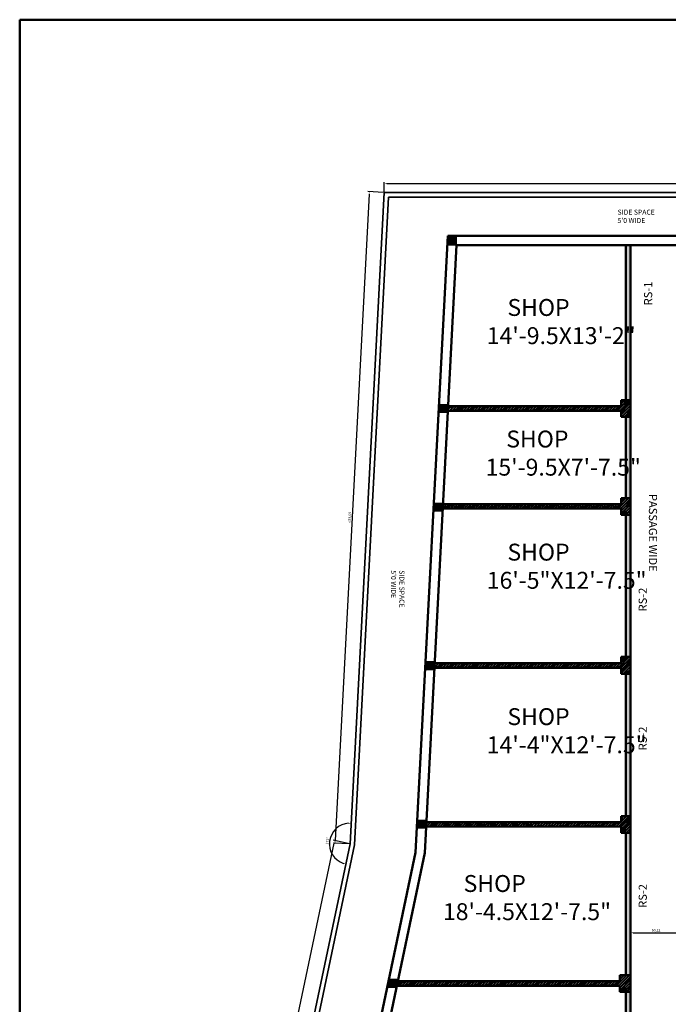
# Model space of a CAD drawing. Units: millimetres. Extents: x 2134 to 3363, y 1052 to 3233.
# Tile 6 of 11: x 2134 to 2770, y 2268 to 3233. Entities that reach past the tile are written whole.
import ezdxf

# ---------------------------------------------------------------- set-up
doc = ezdxf.new("R2010")
doc.units = ezdxf.units.MM
for name, color, linetype, lineweight in [('A-ANNO-DIMS', 2, 'Continuous', 18), ('A-ANNO-TEXT', 7, 'Continuous', 18), ('A-ANNO-TTLB', 7, 'Continuous', 50), ('A-AREA-IDEN', 3, 'Continuous', 18), ('A-COLS', 1, 'Continuous', 35), ('A-WALL', 7, 'Continuous', 50), ('A-WALL-PATT', 8, 'Continuous', 13), ('C-PROP', 6, 'Continuous', 35)]:
    doc.layers.add(name, color=color, linetype=linetype, lineweight=lineweight)
doc.styles.get("Standard").update_dxf_attribs({"font": 'arial.ttf'})
doc.styles.add('YQ_DIM', font='SUPEROS.SHX', dxfattribs={"width": 0.8, "bigfont": 'HZDX.SHX'})
doc.dimstyles.new('ISO-25', dxfattribs={"dimtxt": 2.5, "dimasz": 2.5, "dimexe": 1.25, "dimexo": 0.625, "dimtad": 1, "dimtxsty": 'Standard', "dimcen": 2.5, "dimadec": 0, "dimazin": 0, "dimtfac": 1, "dimtmove": 0, "dimatfit": 3, "dimfxl": 1, "dimarcsym": 0})
pattern_1 = [(45, (2052.4981, 1503.6934), (-1.3470384, 1.3470384), []), (45, (2053.3961, 1503.6934), (-1.3470384, 1.3470384), [])]

# ---------------------------------------------------------------- blocks, each defined once
blk = doc.blocks.new('*D7')
at = {"layer": 'A-ANNO-DIMS', "color": 0, "lineweight": -2, "transparency": 16777216}
for p, q in [((2476.99, 3062.09), (2443.78, 2428.27)), ((2491.22, 3063.85), (2475.87, 3064.66)), ((2457.74, 2425.04), (2442.4, 2425.84))]:
    blk.add_line(p, q, dxfattribs=at)
at = {"layer": 'A-ANNO-DIMS', "color": 0, "transparency": 16777216}
for points in [[(2476.58, 3062.12), (2477.41, 3062.07), (2477.12, 3064.59)], [(2443.36, 2428.3), (2444.19, 2428.25), (2443.64, 2425.78)]]:
    blk.add_solid(points, dxfattribs=at)
at = {"layer": 'Defpoints', "color": 0, "transparency": 16777216}
for p in [(2491.84, 3063.82), (2443.64, 2425.78), (2458.36, 2425.01)]:
    blk.add_point(p, dxfattribs=at)
at = {"layer": 'A-ANNO-DIMS', "color": 0, "transparency": 16777216, "insert": (2458.26, 2745.3), "char_height": 2.5, "attachment_point": 5, "rotation": 87}
blk.add_mtext('639,69', dxfattribs=at)
blk = doc.blocks.new('*D8')
at = {"layer": 'A-ANNO-DIMS', "color": 0, "lineweight": -2, "transparency": 16777216}
for p, q in [((2442.41, 2425.81), (2184.54, 1200.99)), ((2457.75, 2425.14), (2441.71, 2428.51)), ((2198.85, 1195.42), (2182.8, 1198.8))]:
    blk.add_line(p, q, dxfattribs=at)
at = {"layer": 'A-ANNO-DIMS', "color": 0, "transparency": 16777216}
for points in [[(2442.01, 2425.9), (2442.82, 2425.72), (2442.93, 2428.26)], [(2184.14, 1201.07), (2184.95, 1200.9), (2184.03, 1198.54)]]:
    blk.add_solid(points, dxfattribs=at)
at = {"layer": 'Defpoints', "color": 0, "transparency": 16777216}
for p in [(2458.36, 2425.01), (2184.03, 1198.54), (2199.46, 1195.29)]:
    blk.add_point(p, dxfattribs=at)
at = {"layer": 'A-ANNO-DIMS', "color": 0, "transparency": 16777216, "insert": (2311.4, 1813.84), "char_height": 2.5, "attachment_point": 5, "rotation": 78.11076}
blk.add_mtext('1256,67', dxfattribs=at)
blk = doc.blocks.new('*D12')
at = {"layer": 'A-ANNO-DIMS', "color": 0, "lineweight": -2, "transparency": 16777216}
for p, q in [((2733.28, 2333.03), (2733.28, 2339.03)), ((2735.78, 2337.78), (2780.9, 2337.78)), ((2783.4, 2333.03), (2783.4, 2339.03))]:
    blk.add_line(p, q, dxfattribs=at)
at = {"layer": 'A-ANNO-DIMS', "color": 0, "transparency": 16777216}
for points in [[(2735.78, 2338.2), (2735.78, 2337.36), (2733.28, 2337.78)], [(2780.9, 2338.2), (2780.9, 2337.36), (2783.4, 2337.78)]]:
    blk.add_solid(points, dxfattribs=at)
at = {"layer": 'Defpoints', "color": 0, "transparency": 16777216}
for p in [(2783.4, 2337.78), (2733.28, 2332.41), (2783.4, 2332.41)]:
    blk.add_point(p, dxfattribs=at)
at = {"layer": 'A-ANNO-DIMS', "color": 0, "transparency": 16777216, "insert": (2758.34, 2339.91), "char_height": 2.5, "attachment_point": 5}
blk.add_mtext('50,12', dxfattribs=at)
blk = doc.blocks.new('*D16')
at = {"layer": 'A-ANNO-DIMS', "color": 0, "lineweight": -2, "transparency": 16777216}
for p, q in [((2491.84, 3064.45), (2491.84, 3073.74)), ((2494.34, 3072.49), (3166.34, 3072.49)), ((3168.84, 3064.45), (3168.84, 3073.74))]:
    blk.add_line(p, q, dxfattribs=at)
at = {"layer": 'A-ANNO-DIMS', "color": 0, "transparency": 16777216}
for points in [[(2494.34, 3072.9), (2494.34, 3072.07), (2491.84, 3072.49)], [(3166.34, 3072.9), (3166.34, 3072.07), (3168.84, 3072.49)]]:
    blk.add_solid(points, dxfattribs=at)
at = {"layer": 'Defpoints', "color": 0, "transparency": 16777216}
for p in [(3168.84, 3072.49), (2491.84, 3063.82), (3168.84, 3063.82)]:
    blk.add_point(p, dxfattribs=at)
at = {"layer": 'A-ANNO-DIMS', "color": 0, "transparency": 16777216, "insert": (2830.34, 3074.39), "char_height": 2.5, "attachment_point": 5}
blk.add_mtext('677', dxfattribs=at)
blk = doc.blocks.new('*D6')
at = {"layer": 'A-ANNO-DIMS', "color": 0, "lineweight": -2, "transparency": 16777216}
blk.add_arc((2458.36, 2425.01), 20.29, 94.06404, 251.04672, dxfattribs=at)
at = {"layer": 'A-ANNO-DIMS', "color": 0, "transparency": 16777216}
for points in [[(2456.92, 2445.66), (2456.93, 2444.83), (2459.42, 2445.27)], [(2451.88, 2406.22), (2451.66, 2405.42), (2454.18, 2405.15)]]:
    blk.add_solid(points, dxfattribs=at)
at = {"layer": 'Defpoints', "color": 0, "transparency": 16777216}
for p in [(2491.84, 3063.82), (2441.94, 2436.92), (2458.36, 2425.01), (2458.36, 2425.01), (2197.07, 1183.92)]:
    blk.add_point(p, dxfattribs=at)
at = {"layer": 'A-ANNO-DIMS', "color": 0, "transparency": 16777216, "insert": (2436.38, 2427.88), "char_height": 2.5, "attachment_point": 5, "rotation": 82.55538}
blk.add_mtext('171°', dxfattribs=at)

msp = doc.modelspace()

# ---------------------------------------------------------------- hatches: boundary and pattern name
at = {"layer": 'A-COLS'}
h = msp.add_hatch(color=256, dxfattribs=at)
h.dxf.hatch_style = 1
h.paths.add_polyline_path([(2563.182, 3020.694), (2554.182, 3020.694), (2554.182, 3011.694), (2563.182, 3011.694)])
h = msp.add_hatch(color=256, dxfattribs=at)
h.dxf.hatch_style = 1
h.paths.add_polyline_path([(2554.119, 2856.44), (2545.119, 2856.44), (2545.119, 2847.44), (2554.119, 2847.44)])
h = msp.add_hatch(color=256, dxfattribs=at)
h.dxf.hatch_style = 1
h.paths.add_polyline_path([(2548.766, 2759.646), (2539.766, 2759.646), (2539.766, 2750.646), (2548.766, 2750.646)])
h = msp.add_hatch(color=256, dxfattribs=at)
h.dxf.hatch_style = 1
h.paths.add_polyline_path([(2540.736, 2604.242), (2531.736, 2604.242), (2531.736, 2595.242), (2540.736, 2595.242)])
h = msp.add_hatch(color=256, dxfattribs=at)
h.dxf.hatch_style = 1
h.paths.add_polyline_path([(2532.481, 2448.839), (2523.481, 2448.839), (2523.481, 2439.839), (2532.481, 2439.839)])
h = msp.add_hatch(color=256, dxfattribs=at)
h.dxf.hatch_style = 1
h.paths.add_polyline_path([(2504.464, 2292.742), (2495.464, 2292.742), (2495.464, 2283.742), (2504.464, 2283.742)])
at = {"layer": 'A-WALL-PATT'}
h = msp.add_hatch(color=256, dxfattribs=at)
h.dxf.hatch_style = 1
h.paths.add_polyline_path([(2733.282, 2279.774), (2728.782, 2279.774), (2728.782, 2144.774), (2733.282, 2144.774)])
h.paths.add_polyline_path([(2733.282, 2435.778), (2728.782, 2435.778), (2728.782, 2296.274), (2733.282, 2296.274)])
h.paths.add_polyline_path([(2733.282, 2128.274), (2728.782, 2128.274), (2728.782, 1988.794), (2733.282, 1988.794)])
h.paths.add_polyline_path([(2733.282, 1972.299), (2728.782, 1972.299), (2728.782, 1844.774), (2692.782, 1808.774), (2403.682, 1808.774), (2402.735, 1804.274), (2697.282, 1804.274), (2733.282, 1840.274)])
h.paths.add_polyline_path([(2733.282, 2591.847), (2728.782, 2591.847), (2728.782, 2452.274), (2733.282, 2452.276)])
h.paths.add_polyline_path([(2733.282, 2747.554), (2728.782, 2747.554), (2728.782, 2608.342), (2733.282, 2608.342)])
h.paths.add_polyline_path([(2733.282, 2843.718), (2728.782, 2843.718), (2728.782, 2764.049), (2733.282, 2764.049)])
h.paths.add_polyline_path([(2733.282, 3012.274), (2728.782, 3012.274), (2728.782, 2860.213), (2733.282, 2860.213)])
h = msp.add_hatch(dxfattribs=at)
h.set_pattern_fill('ANSI32', color=256, scale=0.2)
h.set_pattern_definition(pattern_1)
h.paths.add_polyline_path([(2733.282, 2860.213), (2728.782, 2860.213), (2724.282, 2860.213), (2724.282, 2854.274), (2554.458, 2854.274), (2554.223, 2849.774), (2724.282, 2849.774), (2724.282, 2843.718), (2728.782, 2843.718), (2733.282, 2843.718)])
h.paths.add_polyline_path([(2733.282, 2764.049), (2728.782, 2764.049), (2724.282, 2764.049), (2724.282, 2758.274), (2549.427, 2758.274), (2549.191, 2753.774), (2724.282, 2753.774), (2724.282, 2747.554), (2728.782, 2747.554), (2733.282, 2747.554)])
h = msp.add_hatch(dxfattribs=at)
h.set_pattern_fill('ANSI32', color=256, scale=0.2)
h.set_pattern_definition(pattern_1)
h.paths.add_polyline_path([(2733.282, 2144.774), (2728.782, 2144.774), (2728.782, 2144.769), (2724.282, 2144.769), (2724.282, 2138.774), (2473.126, 2138.774), (2472.179, 2134.274), (2724.282, 2134.274), (2724.282, 2128.274), (2728.782, 2128.274), (2733.282, 2128.274)])
h.paths.add_polyline_path([(2733.282, 2608.342), (2724.282, 2608.342), (2724.282, 2602.274), (2541.252, 2602.274), (2541.016, 2597.774), (2724.282, 2597.774), (2724.282, 2591.847), (2733.282, 2591.847)])
h.paths.add_polyline_path([(2733.282, 2452.274), (2728.782, 2452.274), (2724.282, 2452.274), (2724.282, 2446.274), (2533.076, 2446.274), (2532.851, 2441.988), (2724.282, 2441.783), (2724.282, 2435.778), (2728.782, 2435.778), (2733.282, 2435.778)])
h.paths.add_polyline_path([(2733.282, 1988.794), (2724.282, 1988.794), (2724.282, 1982.774), (2440.298, 1982.774), (2439.351, 1978.274), (2724.282, 1978.274), (2724.282, 1972.299), (2733.282, 1972.299)])
h.paths.add_polyline_path([(2733.282, 2296.269), (2722.735, 2296.269), (2722.735, 2290.274), (2505.008, 2290.274), (2504.061, 2285.774), (2722.735, 2285.774), (2722.735, 2279.774), (2728.782, 2279.774), (2733.282, 2279.774)])

# ---------------------------------------------------------------- linework, layer by layer
at = {"layer": 'A-ANNO-TTLB', "ltscale": 0.5}
msp.add_lwpolyline([(2134.34, 3233.23), (3362.77, 3233.23), (3362.77, 1152.237), (2134.34, 1152.237)], close=True, dxfattribs=at)
at = {"layer": 'A-WALL'}
for p, q in [((2522.51, 2416.625), (2554.198, 3021.274)), ((2554.198, 3021.274), (3104.339, 3021.274)), ((2575.001, 3021.274), (3104.339, 3021.274)), ((2531.497, 2416.154), (2562.739, 3012.274)), ((2562.739, 3012.274), (3095.339, 3012.274)), ((2567.009, 3012.274), (3095.339, 3012.274)), ((2728.782, 3012.274), (2728.782, 2860.213)), ((2733.282, 3012.274), (2733.282, 1840.274)), ((2724.282, 2854.213), (2724.282, 2860.213)), ((2724.282, 2860.213), (2728.782, 2860.213)), ((2728.782, 2860.213), (2733.282, 2860.213)), ((2554.223, 2849.774), (2724.282, 2849.774)), ((2554.458, 2854.274), (2724.282, 2854.274)), ((2724.282, 2843.718), (2724.282, 2849.774)), ((2728.782, 2843.718), (2724.282, 2843.718)), ((2728.782, 2843.718), (2728.782, 2764.049)), ((2728.782, 2843.718), (2733.282, 2843.718)), ((2724.282, 2758.274), (2724.282, 2764.049)), ((2724.282, 2764.049), (2728.782, 2764.049)), ((2728.782, 2764.049), (2733.282, 2764.049)), ((2549.191, 2753.774), (2724.282, 2753.774)), ((2549.427, 2758.274), (2724.282, 2758.274)), ((2724.282, 2747.554), (2724.282, 2753.774)), ((2728.782, 2747.554), (2724.282, 2747.554)), ((2728.782, 2747.554), (2728.782, 2608.274)), ((2728.782, 2747.554), (2733.282, 2747.554)), ((2724.282, 2602.274), (2724.282, 2608.342)), ((2724.282, 2608.342), (2733.282, 2608.342)), ((2541.016, 2597.774), (2724.282, 2597.774)), ((2541.252, 2602.274), (2724.282, 2602.274)), ((2724.282, 2591.847), (2724.282, 2597.852)), ((2733.282, 2591.847), (2724.282, 2591.847)), ((2728.782, 2591.847), (2728.782, 2452.274)), ((2533.08, 2446.351), (2724.282, 2446.274)), ((2724.282, 2446.274), (2724.282, 2452.274)), ((2724.282, 2452.274), (2728.782, 2452.274)), ((2728.782, 2452.274), (2733.282, 2452.276)), ((2532.851, 2441.988), (2724.282, 2441.783)), ((2724.282, 2435.778), (2724.282, 2441.783)), ((2728.782, 2435.778), (2724.282, 2435.778)), ((2728.782, 2435.778), (2728.782, 2296.274)), ((2728.782, 2435.778), (2733.282, 2435.778)), ((2462.764, 2424.08), (2462.818, 2424.077)), ((2386.865, 1772.344), (2522.51, 2416.625)), ((2396.963, 1776.846), (2531.497, 2416.154)), ((2505.106, 2290.274), (2722.735, 2290.274)), ((2722.735, 2290.269), (2722.735, 2296.269)), ((2722.735, 2296.269), (2733.282, 2296.269)), ((2728.782, 2296.274), (2733.282, 2296.274)), ((2504.158, 2285.774), (2722.735, 2285.774)), ((2722.735, 2279.774), (2722.735, 2285.778)), ((2728.782, 2279.774), (2722.735, 2279.774)), ((2728.782, 2279.774), (2728.782, 2144.769)), ((2728.782, 2279.774), (2733.282, 2279.774))]:
    msp.add_line(p, q, dxfattribs=at)
at = {"layer": 'C-PROP'}
for p, q in [((2458.361, 2425.007), (2491.839, 3063.82)), ((2491.839, 3063.82), (3168.839, 3063.82)), ((2462.817, 2424.049), (2496.11, 3059.32)), ((2496.11, 3059.32), (3164.339, 3059.32)), ((2197.066, 1183.92), (2458.361, 2425.007)), ((2203.596, 1193.093), (2462.764, 2424.08))]:
    msp.add_line(p, q, dxfattribs=at)

# ---------------------------------------------------------------- texts
at = {"layer": 'A-ANNO-TEXT', "char_height": 8, "attachment_point": 1, "rotation": 90, "style": 'YQ_DIM'}
for s, insert in [('{\\fSwis721 BlkCn BT|b0|i0|c0|p34;RS-1}', (2746.589, 2953.097)), ('{\\fSwis721 BlkCn BT|b0|i0|c0|p34;RS-2}', (2741.318, 2652.941)), ('{\\fSwis721 BlkCn BT|b0|i0|c0|p34;RS-2}', (2741.318, 2516.736)), ('{\\fSwis721 BlkCn BT|b0|i0|c0|p34;RS-2}', (2741.318, 2362.301))]:
    msp.add_mtext_dynamic_manual_height_columns(s, width=14.9584, gutter_width=12.5, heights=[0], dxfattribs=dict(at, insert=insert))
at = {"layer": 'A-AREA-IDEN', "attachment_point": 1, "style": 'YQ_DIM'}
for s, width, gutter_width, insert, char_height in [("{\\f@Arial Unicode MS|b0|i0|c134|p34;SIDE SPACE\\P5'0 WIDE}", 92.43125, 24.565, (2720.575, 3046.941), 4.91305), ('{\\f@SimSun|b1|i0|c0|p2; \\f@Arial Unicode MS|b1|i0|c0|p34;   SHOP\\P14\'-9.5X13\'-2\\f@SimSun|b1|i0|c0|p2;"}', 128.94034, 26.518, (2592.365, 2959.304), 16.56819), ('{\\f@SimSun|b1|i0|c0|p2; \\f@Arial Unicode MS|b1|i0|c0|p34;   SHOP\\P15\'-9.5X7\'-7.5\\f@SimSun|b1|i0|c0|p2;"}', 128.94034, 26.518, (2591.238, 2830.309), 16.56819), ('{\\f@SimSun|b1|i0|c0|p2; \\f@Arial Unicode MS|b1|i0|c0|p34;   SHOP\\P16\'-5"X12\'-7.5\\f@SimSun|b1|i0|c0|p2;"}', 128.94034, 26.518, (2592.365, 2719.378), 16.56819), ('{\\f@SimSun|b1|i0|c0|p2; \\f@Arial Unicode MS|b1|i0|c0|p34;   SHOP\\P14\'-4"X12\'-7.5\\f@SimSun|b1|i0|c0|p2;"}', 128.94034, 26.518, (2592.365, 2558.057), 16.56819), ('{\\f@SimSun|b1|i0|c0|p2; \\f@Arial Unicode MS|b1|i0|c0|p34;   SHOP\\P18\'-4.5X12\'-7.5\\f@SimSun|b1|i0|c0|p2;"}', 128.94034, 26.518, (2549.381, 2394.42), 16.56819)]:
    msp.add_mtext_dynamic_manual_height_columns(s, width=width, gutter_width=gutter_width, heights=[0], dxfattribs=dict(at, insert=insert, char_height=char_height))
at = {"layer": 'A-AREA-IDEN', "attachment_point": 1, "rotation": 270, "style": 'YQ_DIM'}
for s, width, gutter_width, insert, char_height in [('\\pxsm2;{\\f@Microsoft YaHei|b0|i0|c0|p34;PASSAGE WIDE}', 84.49104, 12.5, (2759.348, 2768.159), 8), ("{\\f@Arial Unicode MS|b0|i0|c134|p34;SIDE SPACE\\P5'0 WIDE}", 92.43125, 24.565, (2511.596, 2693.242), 4.91305)]:
    msp.add_mtext_dynamic_manual_height_columns(s, width=width, gutter_width=gutter_width, heights=[0], dxfattribs=dict(at, insert=insert, char_height=char_height))

# ---------------------------------------------------------------- dimensions: what is measured, and where the dimension line sits
at = {"layer": 'A-ANNO-DIMS'}
for base, p1, p2, picture, middle in [((3168.839, 3072.486), (2491.839, 3063.82), (3168.839, 3063.82), '*D16', (2830.339, 3074.387)), ((2783.402, 2337.781), (2733.282, 2332.407), (2783.402, 2332.407), '*D12', (2758.342, 2339.909))]:
    dim = msp.add_linear_dim(base=base, p1=p1, p2=p2, dimstyle='ISO-25', override={"dimclrd": 0, "dimclre": 0, "dimclrt": 0}, dxfattribs=at)
    dim.commit()
    dim.dimension.update_dxf_attribs({"geometry": picture, "text_midpoint": middle})
dim = msp.add_angular_dim_2l(base=(2441.938, 2436.923), line1=((2197.066, 1183.92), (2458.361, 2425.007)), line2=((2458.361, 2425.007), (2491.839, 3063.82)), dimstyle='ISO-25', override={"dimclrd": 0, "dimclre": 0, "dimclrt": 0}, dxfattribs=at)
dim.commit()
dim.dimension.update_dxf_attribs({"geometry": '*D6', "text_midpoint": (2436.377, 2427.88)})
for p1, p2, distance, picture, middle in [((2491.839, 3063.82), (2458.361, 2425.007), -14.736, '*D7', (2458.259, 2745.296)), ((2458.361, 2425.007), (2199.46, 1195.291), -15.77, '*D8', (2311.397, 1813.836))]:
    dim = msp.add_aligned_dim(p1=p1, p2=p2, distance=distance, dimstyle='ISO-25', override={"dimclrd": 0, "dimclre": 0, "dimclrt": 0}, dxfattribs=at)
    dim.commit()
    dim.dimension.update_dxf_attribs({"geometry": picture, "text_midpoint": middle})

doc.saveas('drawing.dxf')
